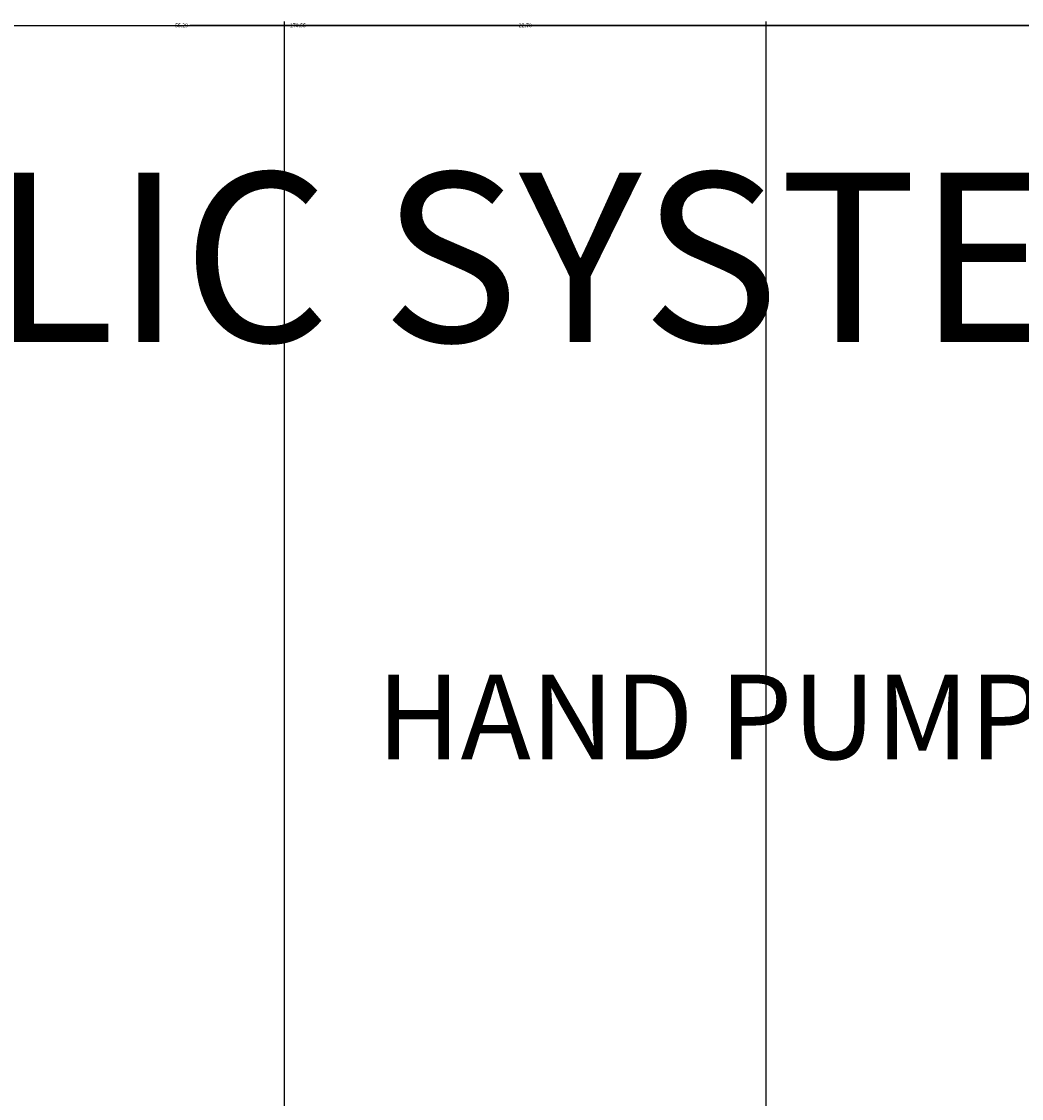
# Model space of a CAD drawing. Units: millimetres. Extents: x -11 to 280, y -4 to 208.
# Tile 47 of 55: x 139 to 186, y 157 to 208. Entities that reach past the tile are written whole.
import ezdxf
from ezdxf import colors
from ezdxf.entities.mleader import LeaderData, LeaderLine
from ezdxf.math import Vec2, Vec3

# ---------------------------------------------------------------- set-up
doc = ezdxf.new("R2010")
doc.units = ezdxf.units.MM
doc.layers.add('M-ANNO-TEXT', color=7, linetype='Continuous', lineweight=18)
doc.layers.add('M-DIMS', color=2, linetype='Continuous', lineweight=18)
doc.styles.get("Standard").update_dxf_attribs({"font": 'arial.ttf'})
doc.dimstyles.get("Standard").update_dxf_attribs({"dimtxt": 0.18, "dimasz": 0.18, "dimexe": 0.18, "dimexo": 0.0625, "dimgap": 0.09, "dimtad": 0, "dimtih": 1, "dimtoh": 1, "dimdec": 4, "dimzin": 0, "dimdsep": 46, "dimtxsty": 'Standard', "dimcen": 0.09, "dimadec": 0, "dimazin": 0, "dimtfac": 1, "dimtdec": 4, "dimtofl": 0, "dimtmove": 0, "dimatfit": 3, "dimfxl": 1, "dimtolj": 1, "dimtzin": 0, "dimarcsym": 0})

# ---------------------------------------------------------------- blocks, each defined once
blk = doc.blocks.new('*D5')
at = {"layer": 'Defpoints', "color": 0, "transparency": 16777216}
for p in [(24.759, 192.645), (-10.087, 11.435), (261.686, 11.435)]:
    blk.add_point(p, dxfattribs=at)
at = {"layer": 'M-DIMS', "color": 0, "lineweight": -2, "transparency": 16777216}
for p, q in [((24.696, 192.645), (-10.267, 192.645)), ((-10.087, 192.465), (-10.087, 102.222)), ((-10.087, 11.615), (-10.087, 101.858)), ((261.624, 11.435), (-10.267, 11.435))]:
    blk.add_line(p, q, dxfattribs=at)
at = {"layer": 'M-DIMS', "color": 0, "transparency": 16777216}
for points in [[(-10.117, 192.465), (-10.057, 192.465), (-10.087, 192.645)], [(-10.117, 11.615), (-10.057, 11.615), (-10.087, 11.435)]]:
    blk.add_solid(points, dxfattribs=at)
at = {"layer": 'M-DIMS', "color": 0, "transparency": 16777216, "insert": (-10.087, 102.04), "char_height": 0.18, "attachment_point": 5}
blk.add_mtext('\\A1;181.2', dxfattribs=at)
blk = doc.blocks.new('*D6')
at = {"layer": 'Defpoints', "color": 0, "transparency": 16777216}
for p in [(236.935, 207.495), (66.388, 179.241), (236.935, 165.103)]:
    blk.add_point(p, dxfattribs=at)
at = {"layer": 'M-DIMS', "color": 0, "lineweight": -2, "transparency": 16777216}
for p, q in [((66.388, 179.304), (66.388, 207.675)), ((66.568, 207.495), (151.206, 207.495)), ((236.755, 207.495), (152.117, 207.495)), ((236.935, 165.166), (236.935, 207.675))]:
    blk.add_line(p, q, dxfattribs=at)
at = {"layer": 'M-DIMS', "color": 0, "transparency": 16777216}
for points in [[(66.568, 207.525), (66.568, 207.465), (66.388, 207.495)], [(236.755, 207.525), (236.755, 207.465), (236.935, 207.495)]]:
    blk.add_solid(points, dxfattribs=at)
at = {"layer": 'M-DIMS', "color": 0, "transparency": 16777216, "insert": (151.661, 207.495), "char_height": 0.18, "attachment_point": 5}
blk.add_mtext('\\A1;170.55', dxfattribs=at)
blk = doc.blocks.new('*D12')
at = {"layer": 'Defpoints', "color": 0, "transparency": 16777216}
for p in [(173.804, 207.495), (118.514, 96.485), (173.804, 89.387)]:
    blk.add_point(p, dxfattribs=at)
at = {"layer": 'M-DIMS', "color": 0, "lineweight": -2, "transparency": 16777216}
for p, q in [((118.514, 96.547), (118.514, 207.675)), ((118.694, 207.495), (145.765, 207.495)), ((173.624, 207.495), (146.553, 207.495)), ((173.804, 89.45), (173.804, 207.675))]:
    blk.add_line(p, q, dxfattribs=at)
at = {"layer": 'M-DIMS', "color": 0, "transparency": 16777216}
for points in [[(118.694, 207.525), (118.694, 207.465), (118.514, 207.495)], [(173.624, 207.525), (173.624, 207.465), (173.804, 207.495)]]:
    blk.add_solid(points, dxfattribs=at)
at = {"layer": 'M-DIMS', "color": 0, "transparency": 16777216, "insert": (146.159, 207.495), "char_height": 0.18, "attachment_point": 5}
blk.add_mtext('\\A1;55.29', dxfattribs=at)
blk = doc.blocks.new('*D18')
at = {"layer": 'Defpoints', "color": 0, "transparency": 16777216}
for p in [(173.804, 207.495), (173.804, 65.064), (151.022, 43.599)]:
    blk.add_point(p, dxfattribs=at)
at = {"layer": 'M-DIMS', "color": 0, "lineweight": -2, "transparency": 16777216}
for p, q in [((151.022, 43.662), (151.022, 207.675)), ((151.202, 207.495), (162.017, 207.495)), ((173.624, 207.495), (162.808, 207.495)), ((173.804, 65.126), (173.804, 207.675))]:
    blk.add_line(p, q, dxfattribs=at)
at = {"layer": 'M-DIMS', "color": 0, "transparency": 16777216}
for points in [[(151.202, 207.525), (151.202, 207.465), (151.022, 207.495)], [(173.624, 207.525), (173.624, 207.465), (173.804, 207.495)]]:
    blk.add_solid(points, dxfattribs=at)
at = {"layer": 'M-DIMS', "color": 0, "transparency": 16777216, "insert": (162.413, 207.495), "char_height": 0.18, "attachment_point": 5}
blk.add_mtext('\\A1;22.78', dxfattribs=at)
blk = doc.blocks.new('*D20')
at = {"layer": 'Defpoints', "color": 0, "transparency": 16777216}
for p in [(231.68, 207.495), (151.022, 43.599), (231.68, 43.599)]:
    blk.add_point(p, dxfattribs=at)
at = {"layer": 'M-DIMS', "color": 0, "lineweight": -2, "transparency": 16777216}
for p, q in [((151.022, 43.662), (151.022, 207.675)), ((151.202, 207.495), (190.957, 207.495)), ((231.5, 207.495), (191.745, 207.495)), ((231.68, 43.662), (231.68, 207.675))]:
    blk.add_line(p, q, dxfattribs=at)
at = {"layer": 'M-DIMS', "color": 0, "transparency": 16777216}
for points in [[(151.202, 207.525), (151.202, 207.465), (151.022, 207.495)], [(231.5, 207.525), (231.5, 207.465), (231.68, 207.495)]]:
    blk.add_solid(points, dxfattribs=at)
at = {"layer": 'M-DIMS', "color": 0, "transparency": 16777216, "insert": (191.351, 207.495), "char_height": 0.18, "attachment_point": 5}
blk.add_mtext('\\A1;80.66', dxfattribs=at)

msp = doc.modelspace()

# ---------------------------------------------------------------- texts
at = {"layer": 'M-ANNO-TEXT', "insert": (94.3946, 200.5299), "char_height": 8, "attachment_point": 1}
msp.add_mtext_dynamic_manual_height_columns('HYDRAULIC SYSTEM ', width=219.105197, gutter_width=12.5, heights=[0], dxfattribs=at)

# ---------------------------------------------------------------- dimensions: what is measured, and where the dimension line sits
at = {"layer": 'M-DIMS'}
for base, p1, p2, picture, middle in [((236.9353, 207.495), (66.3875, 179.2412), (236.9353, 165.103), '*D6', (151.6614, 207.495)), ((173.8038, 207.495), (118.5137, 96.4849), (173.8038, 89.3873), '*D12', (146.1587, 207.495)), ((173.8038, 207.495), (151.0217, 43.5991), (173.8038, 65.0638), '*D18', (162.4127, 207.495)), ((231.6803, 207.495), (151.0217, 43.5991), (231.6803, 43.5991), '*D20', (191.351, 207.495))]:
    dim = msp.add_linear_dim(base=base, p1=p1, p2=p2, dimstyle='Standard', override={"dimdec": 2, "dimlfac": 1, "dimrnd": 0, "dimzin": 0, "dimdsep": 46, "dimlunit": 2}, dxfattribs=at)
    dim.commit()
    dim.dimension.update_dxf_attribs({"geometry": picture, "text_midpoint": middle})
dim = msp.add_linear_dim(base=(-10.0865, 11.4346), p1=(24.7588, 192.645), p2=(261.6863, 11.4346), angle=90, dimstyle='Standard', override={"dimdec": 1, "dimlfac": 1, "dimrnd": 0, "dimzin": 0, "dimdsep": 46, "dimlunit": 2}, dxfattribs=at)
dim.commit()
dim.dimension.update_dxf_attribs({"geometry": '*D5', "text_midpoint": (-10.0865, 102.0398)})

# ---------------------------------------------------------------- leaders
at = {"layer": 'M-ANNO-TEXT'}
ml = msp.add_multileader_mtext('Standard', dxfattribs=at)
ml.set_content('HAND PUMP', color=256)
ml.set_leader_properties()
ml.build(insert=Vec2(0, 0))
ctx = ml.context
ctx.base_point, ctx.plane_origin = Vec3(152.0312, 174.7629), Vec3(205.5315, 166.103)
ctx.text_align_type = 2
notes = []
notes.append((ctx, [(0, (1, 1, 0), (196.8716, 174.7629), (-1, 0), 8, [(0, [(205.5315, 166.103)], 0, [])])]))
ctx.mtext.insert, ctx.mtext.alignment, ctx.mtext.flow_direction = Vec3(186.8716, 176.7971), 3, 5
for ctx, leaders in notes:
    for number, flags, end, landing, length, lines in leaders:
        leader = LeaderData()
        leader.index, (leader.has_last_leader_line, leader.has_dogleg_vector, leader.attachment_direction) = number, flags
        leader.last_leader_point, leader.dogleg_vector, leader.dogleg_length = Vec3(end), Vec3(landing), length
        for number, points, colour, breaks in lines:
            line = LeaderLine()
            line.index, line.vertices, line.color, line.breaks = number, Vec3.list(points), colors.encode_raw_color(colour), breaks
            leader.lines.append(line)
        ctx.leaders.append(leader)

doc.saveas('drawing.dxf')
